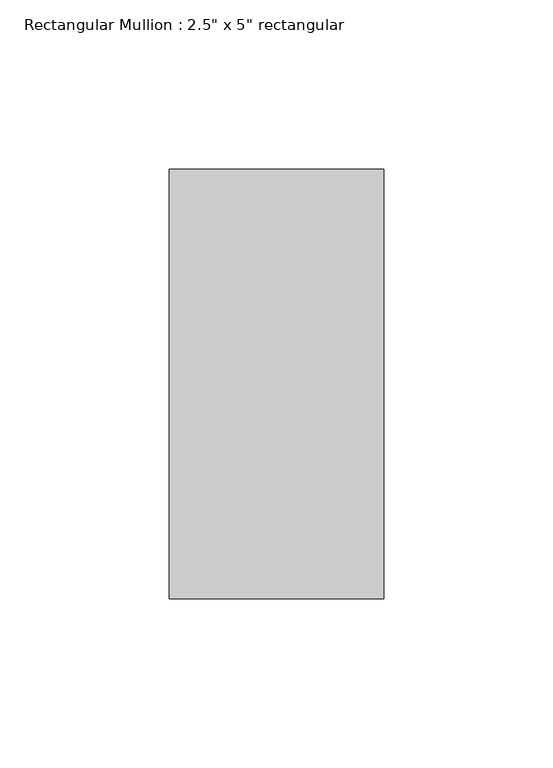
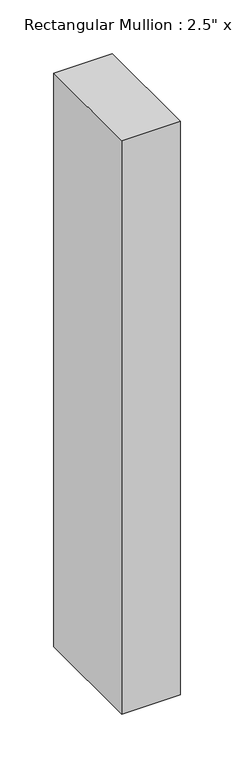
"""IFC4 building model written with IfcOpenShell, lengths in millimetres: member geometry."""

from ifc_helpers import new_model, si_unit, frame, origin, place, context, project, spatial, polyline, outline, extrude, source, transform, mapped, element, save


def member_e51dd2bd(model_context):
    return source(origin(), model_context, "Body", "SweptSolid", [
        extrude(outline(polyline([(31.75, 63.5), (31.75, -63.5), (-31.75, -63.5), (-31.75, 63.5), (31.75, 63.5)])), frame((0.0, 0.0, -654.1955358), z_axis=(0.0, 0.0, 1.0), x_axis=(1.0, 0.0, 0.0)), (0.0, 0.0, 1.0), 654.1955358),
    ])


if __name__ == "__main__":
    model = new_model("IFC4")
    model_context = context("Model", 3, world=origin())
    ifc_project = project(units=[si_unit("LENGTHUNIT", "METRE", prefix="MILLI")], contexts=[model_context])
    site = spatial("IfcSite", under=ifc_project)
    building = spatial("IfcBuilding", under=site)
    placement = place(None, origin())
    member_shape = member_e51dd2bd(model_context)
    element("IfcMember", 1, ObjectType="Rectangular Mullion : 2.5\" x 5\" rectangular", at=placement, inside=building, context=model_context, shape_type="MappedRepresentation", body=[
        mapped(member_shape, transform((0.0, 0.0, 0.0), x_axis=(1.0, 0.0, 0.0), y_axis=(0.0, 1.0, 0.0), z_axis=(0.0, 0.0, 1.0))),
    ])
    save(model, "model.ifc")

# Revit data of these elements
# Type "Rectangular Mullion : 2.5\" x 5\" rectangular"
#   built-in parameter 1007304 = 0.416667 (stored number, unit not read)
#   built-in parameter 1007301 = 0.104167 (stored number, unit not read)
#   built-in parameter 1007300 = 0.104167 (stored number, unit not read)
# Element 1 (IfcMember, "Rectangular Mullion : 2.5\" x 5\" rectangular")
#   Materials on its faces: "Aluminum"
# Materials
#   "Aluminum": class "Metal", colour RGB 247 247 247, transparency 0, Description = "Aluminum 6061", Cost = 0
